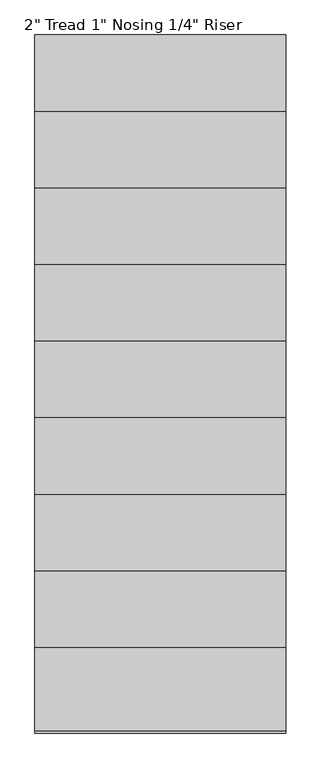
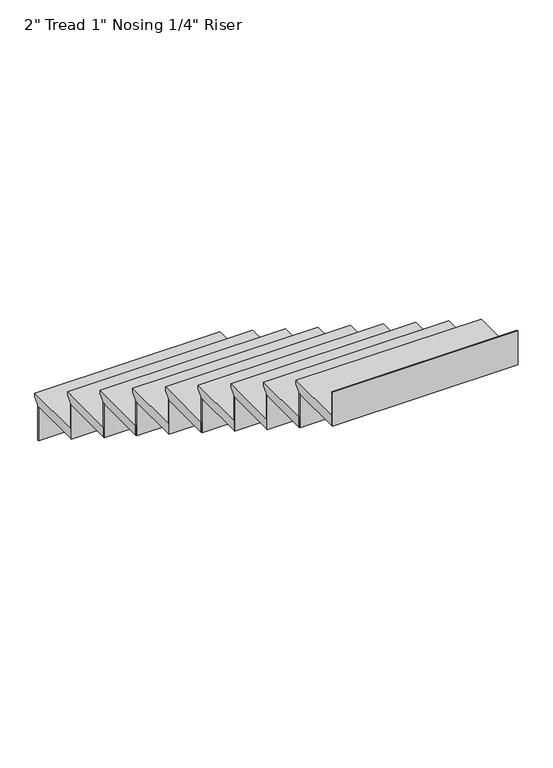
"""IFC4 building model written with IfcOpenShell, lengths in millimetres: stair flight geometry."""

from ifc_helpers import new_model, si_unit, frame, origin, place, context, project, spatial, polyline, outline, extrude, source, transform, mapped, element, save


def stair_flight_50bec54b(model_context):
    return source(origin(), model_context, "Body", "SweptSolid", [
        extrude(outline(polyline([(1808.6257925, 2209.8), (2113.4257925, 2209.8), (2113.4257925, 2190.75), (2088.0257925, 2165.35), (2088.0257925, 2159.0), (1808.6257925, 2159.0), (1808.6257925, 2209.8)])), frame((1465.4501403, 0.0, 0.0), z_axis=(1.0, 0.0, 0.0), x_axis=(0.0, 1.0, 0.0)), (0.0, 0.0, 1.0), 914.4),
        extrude(outline(polyline([(1465.4501403, 2081.6757925), (1465.4501403, 2088.0257925), (2379.8501403, 2088.0257925), (2379.8501403, 2081.6757925), (1465.4501403, 2081.6757925)])), frame((0.0, 0.0, 1981.2), z_axis=(0.0, 0.0, 1.0), x_axis=(1.0, 0.0, 0.0)), (0.0, 0.0, 1.0), 177.8),
        extrude(outline(polyline([(1465.4501403, 1802.2757925), (1465.4501403, 1808.6257925), (2379.8501403, 1808.6257925), (2379.8501403, 1802.2757925), (1465.4501403, 1802.2757925)])), frame((0.0, 0.0, 2159.0), z_axis=(0.0, 0.0, 1.0), x_axis=(1.0, 0.0, 0.0)), (0.0, 0.0, 1.0), 177.8),
        extrude(outline(polyline([(1529.2257925, 2387.6), (1834.0257925, 2387.6), (1834.0257925, 2368.55), (1808.6257925, 2343.15), (1808.6257925, 2336.8), (1529.2257925, 2336.8), (1529.2257925, 2387.6)])), frame((1465.4501403, 0.0, 0.0), z_axis=(1.0, 0.0, 0.0), x_axis=(0.0, 1.0, 0.0)), (0.0, 0.0, 1.0), 914.4),
        extrude(outline(polyline([(1465.4501403, 1522.8757925), (1465.4501403, 1529.2257925), (2379.8501403, 1529.2257925), (2379.8501403, 1522.8757925), (1465.4501403, 1522.8757925)])), frame((0.0, 0.0, 2336.8), z_axis=(0.0, 0.0, 1.0), x_axis=(1.0, 0.0, 0.0)), (0.0, 0.0, 1.0), 177.8),
        extrude(outline(polyline([(1249.8257925, 2565.4), (1554.6257925, 2565.4), (1554.6257925, 2546.35), (1529.2257925, 2520.95), (1529.2257925, 2514.6), (1249.8257925, 2514.6), (1249.8257925, 2565.4)])), frame((1465.4501403, 0.0, 0.0), z_axis=(1.0, 0.0, 0.0), x_axis=(0.0, 1.0, 0.0)), (0.0, 0.0, 1.0), 914.4),
        extrude(outline(polyline([(1465.4501403, 1243.4757925), (1465.4501403, 1249.8257925), (2379.8501403, 1249.8257925), (2379.8501403, 1243.4757925), (1465.4501403, 1243.4757925)])), frame((0.0, 0.0, 2514.6), z_axis=(0.0, 0.0, 1.0), x_axis=(1.0, 0.0, 0.0)), (0.0, 0.0, 1.0), 177.8),
        extrude(outline(polyline([(970.4257925, 2743.2), (1275.2257925, 2743.2), (1275.2257925, 2724.15), (1249.8257925, 2698.75), (1249.8257925, 2692.4), (970.4257925, 2692.4), (970.4257925, 2743.2)])), frame((1465.4501403, 0.0, 0.0), z_axis=(1.0, 0.0, 0.0), x_axis=(0.0, 1.0, 0.0)), (0.0, 0.0, 1.0), 914.4),
        extrude(outline(polyline([(1465.4501403, 964.0757925), (1465.4501403, 970.4257925), (2379.8501403, 970.4257925), (2379.8501403, 964.0757925), (1465.4501403, 964.0757925)])), frame((0.0, 0.0, 2692.4), z_axis=(0.0, 0.0, 1.0), x_axis=(1.0, 0.0, 0.0)), (0.0, 0.0, 1.0), 177.8),
        extrude(outline(polyline([(691.0257925, 2921.0), (995.8257925, 2921.0), (995.8257925, 2901.95), (970.4257925, 2876.55), (970.4257925, 2870.2), (691.0257925, 2870.2), (691.0257925, 2921.0)])), frame((1465.4501403, 0.0, 0.0), z_axis=(1.0, 0.0, 0.0), x_axis=(0.0, 1.0, 0.0)), (0.0, 0.0, 1.0), 914.4),
        extrude(outline(polyline([(1465.4501403, 684.6757925), (1465.4501403, 691.0257925), (2379.8501403, 691.0257925), (2379.8501403, 684.6757925), (1465.4501403, 684.6757925)])), frame((0.0, 0.0, 2870.2), z_axis=(0.0, 0.0, 1.0), x_axis=(1.0, 0.0, 0.0)), (0.0, 0.0, 1.0), 177.8),
        extrude(outline(polyline([(411.6257925, 3098.8), (716.4257925, 3098.8), (716.4257925, 3079.75), (691.0257925, 3054.35), (691.0257925, 3048.0), (411.6257925, 3048.0), (411.6257925, 3098.8)])), frame((1465.4501403, 0.0, 0.0), z_axis=(1.0, 0.0, 0.0), x_axis=(0.0, 1.0, 0.0)), (0.0, 0.0, 1.0), 914.4),
        extrude(outline(polyline([(1465.4501403, 405.2757925), (1465.4501403, 411.6257925), (2379.8501403, 411.6257925), (2379.8501403, 405.2757925), (1465.4501403, 405.2757925)])), frame((0.0, 0.0, 3048.0), z_axis=(0.0, 0.0, 1.0), x_axis=(1.0, 0.0, 0.0)), (0.0, 0.0, 1.0), 177.8),
        extrude(outline(polyline([(132.2257925, 3276.6), (437.0257925, 3276.6), (437.0257925, 3257.55), (411.6257925, 3232.15), (411.6257925, 3225.8), (132.2257925, 3225.8), (132.2257925, 3276.6)])), frame((1465.4501403, 0.0, 0.0), z_axis=(1.0, 0.0, 0.0), x_axis=(0.0, 1.0, 0.0)), (0.0, 0.0, 1.0), 914.4),
        extrude(outline(polyline([(1465.4501403, 125.8757925), (1465.4501403, 132.2257925), (2379.8501403, 132.2257925), (2379.8501403, 125.8757925), (1465.4501403, 125.8757925)])), frame((0.0, 0.0, 3225.8), z_axis=(0.0, 0.0, 1.0), x_axis=(1.0, 0.0, 0.0)), (0.0, 0.0, 1.0), 177.8),
        extrude(outline(polyline([(-147.1742075, 3454.4), (157.6257925, 3454.4), (157.6257925, 3435.35), (132.2257925, 3409.95), (132.2257925, 3403.6), (-147.1742075, 3403.6), (-147.1742075, 3454.4)])), frame((1465.4501403, 0.0, 0.0), z_axis=(1.0, 0.0, 0.0), x_axis=(0.0, 1.0, 0.0)), (0.0, 0.0, 1.0), 914.4),
        extrude(outline(polyline([(1465.4501403, -153.5242075), (1465.4501403, -147.1742075), (2379.8501403, -147.1742075), (2379.8501403, -153.5242075), (1465.4501403, -153.5242075)])), frame((0.0, 0.0, 3403.6), z_axis=(0.0, 0.0, 1.0), x_axis=(1.0, 0.0, 0.0)), (0.0, 0.0, 1.0), 177.8),
        extrude(outline(polyline([(1465.4501403, -432.9242075), (1465.4501403, -426.5742075), (2379.8501403, -426.5742075), (2379.8501403, -432.9242075), (1465.4501403, -432.9242075)])), frame((0.0, 0.0, 3581.4), z_axis=(0.0, 0.0, 1.0), x_axis=(1.0, 0.0, 0.0)), (0.0, 0.0, 1.0), 177.8),
        extrude(outline(polyline([(-426.5742075, 3632.2), (-121.7742075, 3632.2), (-121.7742075, 3613.15), (-147.1742075, 3587.75), (-147.1742075, 3581.4), (-426.5742075, 3581.4), (-426.5742075, 3632.2)])), frame((1465.4501403, 0.0, 0.0), z_axis=(1.0, 0.0, 0.0), x_axis=(0.0, 1.0, 0.0)), (0.0, 0.0, 1.0), 914.4),
    ])


if __name__ == "__main__":
    model = new_model("IFC4")
    model_context = context("Model", 3, world=origin())
    ifc_project = project(units=[si_unit("LENGTHUNIT", "METRE", prefix="MILLI")], contexts=[model_context])
    site = spatial("IfcSite", under=ifc_project)
    building = spatial("IfcBuilding", under=site)
    placement = place(None, origin())
    stair_flight_shape = stair_flight_50bec54b(model_context)
    element("IfcStairFlight", 1, ObjectType="2\" Tread 1\" Nosing 1/4\" Riser", at=placement, inside=building, context=model_context, shape_type="MappedRepresentation", body=[
        mapped(stair_flight_shape, transform((0.0, 0.0, 0.0), x_axis=(1.0, 0.0, 0.0), y_axis=(0.0, 1.0, 0.0), z_axis=(0.0, 0.0, 1.0))),
    ])
    save(model, "model.ifc")
